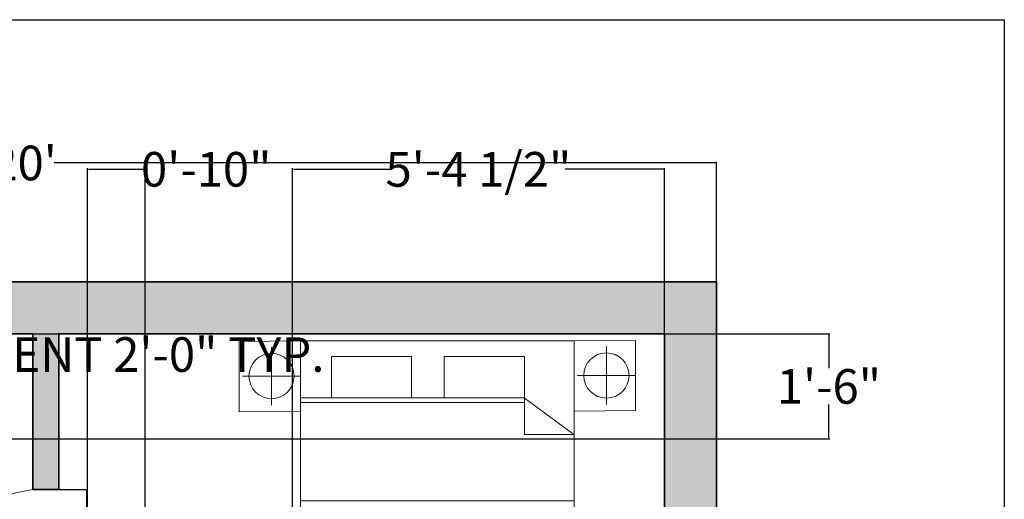
# Model space of a CAD drawing. Units: inches. Extents: x 335 to 688, y 1043 to 1486.
# Tile 7 of 7: x 510 to 681, y 1403 to 1486. Entities that reach past the tile are written whole.
import ezdxf

# ---------------------------------------------------------------- set-up
doc = ezdxf.new("R2010")
doc.units = ezdxf.units.IN
doc.header["$MEASUREMENT"] = 0
for name, color, linetype, lineweight in [('A-ANNO-DIMS', 2, 'Continuous', 18), ('A-ANNO-TTLB', 7, 'Continuous', 25), ('A-DOOR', 4, 'Continuous', 18), ('A-FURN', 8, 'Continuous', 18), ('A-WALL', 7, 'Continuous', 35), ('A-WALL-PATT', 252, 'Continuous', 13)]:
    doc.layers.add(name, color=color, linetype=linetype, lineweight=lineweight)
doc.styles.get("Standard").update_dxf_attribs({"font": 'arial.ttf'})
doc.dimstyles.get("Standard").update_dxf_attribs({"dimtxt": 6, "dimasz": 0.18, "dimexe": 0.18, "dimexo": 0.0625, "dimgap": 0.09, "dimtad": 0, "dimtih": 1, "dimtoh": 1, "dimdec": 1, "dimzin": 0, "dimdsep": 46, "dimlunit": 3, "dimtxsty": 'Standard', "dimcen": 0.09, "dimadec": 0, "dimazin": 0, "dimtfac": 1, "dimtdec": 1, "dimtofl": 0, "dimtmove": 0, "dimatfit": 3, "dimfxl": 1, "dimtolj": 1, "dimtzin": 0, "dimarcsym": 0})

# ---------------------------------------------------------------- blocks, each defined once
blk = doc.blocks.new('*D3')
at = {"layer": 'A-ANNO-DIMS', "color": 0, "lineweight": -2, "transparency": 16777216}
for p, q in [((391.11, 1441.03), (391.11, 1461.75)), ((391.29, 1461.57), (505.87, 1461.57)), ((630.93, 1461.57), (516.34, 1461.57)), ((631.11, 1441.03), (631.11, 1461.75))]:
    blk.add_line(p, q, dxfattribs=at)
at = {"layer": 'A-ANNO-DIMS', "color": 0, "transparency": 16777216}
for points in [[(391.29, 1461.6), (391.29, 1461.54), (391.11, 1461.57)], [(630.93, 1461.6), (630.93, 1461.54), (631.11, 1461.57)]]:
    blk.add_solid(points, dxfattribs=at)
at = {"layer": 'Defpoints', "color": 0, "transparency": 16777216}
for p in [(631.11, 1461.57), (391.11, 1440.97), (631.11, 1440.97)]:
    blk.add_point(p, dxfattribs=at)
at = {"layer": 'A-ANNO-DIMS', "color": 0, "transparency": 16777216, "insert": (511.11, 1461.57), "char_height": 6, "attachment_point": 5}
blk.add_mtext("\\A1;20'", dxfattribs=at)
blk = doc.blocks.new('BED-DOUBLE-WITH-NIGHTSTANDS')
for p, q in [((56.59, 58.08), (56.59, 68.14)), ((0, 64.35), (26.37, 64.35)), ((0, 1.12), (0, 64.35)), ((26.37, 64.35), (26.37, 58.06)), ((61.62, 63.11), (51.56, 63.11)), ((34.96, 10.66), (34.96, 58.08)), ((52, 19.27), (52, 58.08)), ((52.82, 19.32), (52.82, 58.08)), ((52.82, 19.32), (46.47, 10.71)), ((52.82, 19.27), (46.47, 19.27)), ((46.47, 19.27), (46.47, 10.71)), ((26.37, 10.66), (26.37, 1.12)), ((56.69, 0.03), (56.69, 10.09)), ((61.72, 5.06), (51.66, 5.06)), ((26.37, 1.12), (0, 1.12))]:
    blk.add_line(p, q)
for points in [[(50.39, 68.71), (50.5, 58.08), (62.68, 58.08), (62.58, 68.71)], [(62.68, 10.66), (11.37, 10.66), (11.37, 58.08), (62.68, 58.08)], [(59.98, 38.83), (52.82, 38.83), (52.82, 52.73), (59.98, 52.73)], [(59.98, 19.27), (52.82, 19.27), (52.82, 33.16), (59.98, 33.16)], [(50.5, 10.66), (50.6, 0.03), (62.78, 0.03), (62.68, 10.66)]]:
    blk.add_lwpolyline(points, close=True)
for centre in [(56.59, 63.11), (56.69, 5.06)]:
    blk.add_circle(centre, 3.92)
for points, knots in [([(0.07, 65.48), (0.19, 65.39), (0.43, 65.19), (0.19, 64.85), (0.02, 64.57), (0.13, 64.42), (0.18, 64.35)], [0, 0, 0, 0, 0.400747, 0.791423, 1.067667, 1.29709, 1.29709, 1.29709, 1.29709]), ([(0.57, 65.48), (0.7, 65.39), (0.94, 65.19), (0.7, 64.85), (0.52, 64.57), (0.63, 64.42), (0.68, 64.35)], [0, 0, 0, 0, 0.400747, 0.791423, 1.067667, 1.29709, 1.29709, 1.29709, 1.29709]), ([(1.06, 65.48), (1.18, 65.39), (1.42, 65.19), (1.18, 64.85), (1.01, 64.57), (1.11, 64.42), (1.16, 64.35)], [0, 0, 0, 0, 0.400747, 0.791423, 1.067667, 1.29709, 1.29709, 1.29709, 1.29709]), ([(1.46, 65.48), (1.58, 65.39), (1.82, 65.19), (1.58, 64.85), (1.41, 64.57), (1.51, 64.42), (1.56, 64.35)], [0, 0, 0, 0, 0.400747, 0.791423, 1.067667, 1.29709, 1.29709, 1.29709, 1.29709]), ([(1.88, 65.48), (2, 65.39), (2.24, 65.19), (2, 64.85), (1.82, 64.57), (1.93, 64.42), (1.98, 64.35)], [0, 0, 0, 0, 0.400747, 0.791423, 1.067667, 1.29709, 1.29709, 1.29709, 1.29709]), ([(2.18, 65.48), (2.31, 65.39), (2.55, 65.19), (2.31, 64.85), (2.13, 64.57), (2.24, 64.42), (2.29, 64.35)], [0, 0, 0, 0, 0.400747, 0.791423, 1.067667, 1.29709, 1.29709, 1.29709, 1.29709]), ([(2.76, 65.48), (2.88, 65.39), (3.12, 65.19), (2.88, 64.85), (2.71, 64.57), (2.81, 64.42), (2.86, 64.35)], [0, 0, 0, 0, 0.400747, 0.791423, 1.067667, 1.29709, 1.29709, 1.29709, 1.29709]), ([(3.33, 65.48), (3.45, 65.39), (3.7, 65.19), (3.44, 64.85), (3.27, 64.57), (3.38, 64.42), (3.43, 64.35)], [0, 0, 0, 0, 0.407265, 0.802015, 1.07826, 1.307683, 1.307683, 1.307683, 1.307683]), ([(3.75, 65.48), (3.88, 65.39), (4.12, 65.19), (3.88, 64.85), (3.7, 64.57), (3.81, 64.42), (3.86, 64.35)], [0, 0, 0, 0, 0.400747, 0.791423, 1.067667, 1.29709, 1.29709, 1.29709, 1.29709]), ([(4.64, 65.48), (4.76, 65.39), (5, 65.19), (4.76, 64.85), (4.59, 64.57), (4.69, 64.42), (4.74, 64.35)], [0, 0, 0, 0, 0.400747, 0.791423, 1.067667, 1.29709, 1.29709, 1.29709, 1.29709]), ([(5.36, 65.48), (5.49, 65.39), (5.73, 65.19), (5.49, 64.85), (5.31, 64.57), (5.42, 64.42), (5.47, 64.35)], [0, 0, 0, 0, 0.400747, 0.791423, 1.067667, 1.29709, 1.29709, 1.29709, 1.29709]), ([(6.12, 65.48), (6.24, 65.39), (6.48, 65.19), (6.24, 64.85), (6.07, 64.57), (6.17, 64.42), (6.22, 64.35)], [0, 0, 0, 0, 0.400747, 0.791423, 1.067667, 1.29709, 1.29709, 1.29709, 1.29709]), ([(7, 65.48), (7.12, 65.39), (7.36, 65.19), (7.12, 64.85), (6.95, 64.57), (7.05, 64.42), (7.1, 64.35)], [0, 0, 0, 0, 0.400747, 0.791423, 1.067667, 1.29709, 1.29709, 1.29709, 1.29709]), ([(7.73, 65.48), (7.85, 65.39), (8.09, 65.19), (7.85, 64.85), (7.68, 64.57), (7.78, 64.42), (7.83, 64.35)], [0, 0, 0, 0, 0.400747, 0.791423, 1.067667, 1.29709, 1.29709, 1.29709, 1.29709]), ([(8.54, 65.48), (8.66, 65.39), (8.9, 65.19), (8.66, 64.85), (8.49, 64.57), (8.6, 64.42), (8.65, 64.35)], [0, 0, 0, 0, 0.400747, 0.791423, 1.067667, 1.29709, 1.29709, 1.29709, 1.29709]), ([(9.23, 65.48), (9.35, 65.39), (9.59, 65.19), (9.35, 64.85), (9.18, 64.57), (9.29, 64.42), (9.34, 64.35)], [0, 0, 0, 0, 0.400747, 0.791423, 1.067667, 1.29709, 1.29709, 1.29709, 1.29709]), ([(10.05, 65.48), (10.17, 65.39), (10.41, 65.19), (10.17, 64.85), (10, 64.57), (10.1, 64.42), (10.15, 64.35)], [0, 0, 0, 0, 0.400747, 0.791423, 1.067667, 1.29709, 1.29709, 1.29709, 1.29709]), ([(10.93, 65.48), (11.05, 65.39), (11.29, 65.19), (11.05, 64.85), (10.88, 64.57), (10.99, 64.42), (11.03, 64.35)], [0, 0, 0, 0, 0.400747, 0.791423, 1.067667, 1.29709, 1.29709, 1.29709, 1.29709]), ([(11.97, 65.48), (12.09, 65.39), (12.33, 65.19), (12.09, 64.85), (11.92, 64.57), (12.02, 64.42), (12.07, 64.35)], [0, 0, 0, 0, 0.400747, 0.791423, 1.067667, 1.29709, 1.29709, 1.29709, 1.29709]), ([(12.85, 65.48), (12.97, 65.39), (13.21, 65.19), (12.97, 64.85), (12.8, 64.57), (12.9, 64.42), (12.95, 64.35)], [0, 0, 0, 0, 0.400747, 0.791423, 1.067667, 1.29709, 1.29709, 1.29709, 1.29709]), ([(13.58, 65.48), (13.7, 65.39), (13.94, 65.19), (13.7, 64.85), (13.53, 64.57), (13.63, 64.42), (13.68, 64.35)], [0, 0, 0, 0, 0.400747, 0.791423, 1.067667, 1.29709, 1.29709, 1.29709, 1.29709]), ([(14.33, 65.48), (14.45, 65.39), (14.69, 65.19), (14.45, 64.85), (14.28, 64.57), (14.38, 64.42), (14.43, 64.35)], [0, 0, 0, 0, 0.400747, 0.791423, 1.067667, 1.29709, 1.29709, 1.29709, 1.29709]), ([(15.21, 65.48), (15.33, 65.39), (15.57, 65.19), (15.33, 64.85), (15.16, 64.57), (15.27, 64.42), (15.32, 64.35)], [0, 0, 0, 0, 0.400747, 0.791423, 1.067667, 1.29709, 1.29709, 1.29709, 1.29709]), ([(15.94, 65.48), (16.06, 65.39), (16.3, 65.19), (16.06, 64.85), (15.89, 64.57), (16, 64.42), (16.04, 64.35)], [0, 0, 0, 0, 0.400747, 0.791423, 1.067667, 1.29709, 1.29709, 1.29709, 1.29709]), ([(16.76, 65.48), (16.88, 65.39), (17.12, 65.19), (16.88, 64.85), (16.7, 64.57), (16.81, 64.42), (16.86, 64.35)], [0, 0, 0, 0, 0.400747, 0.791423, 1.067667, 1.29709, 1.29709, 1.29709, 1.29709]), ([(17.53, 65.48), (17.65, 65.39), (17.89, 65.19), (17.65, 64.85), (17.48, 64.57), (17.59, 64.42), (17.64, 64.35)], [0, 0, 0, 0, 0.400747, 0.791423, 1.067667, 1.29709, 1.29709, 1.29709, 1.29709]), ([(18.35, 65.48), (18.47, 65.39), (18.71, 65.19), (18.47, 64.85), (18.3, 64.57), (18.4, 64.42), (18.45, 64.35)], [0, 0, 0, 0, 0.400747, 0.791423, 1.067667, 1.29709, 1.29709, 1.29709, 1.29709]), ([(19.23, 65.48), (19.35, 65.39), (19.59, 65.19), (19.35, 64.85), (19.18, 64.57), (19.29, 64.42), (19.33, 64.35)], [0, 0, 0, 0, 0.400747, 0.791423, 1.067667, 1.29709, 1.29709, 1.29709, 1.29709]), ([(20.27, 65.48), (20.39, 65.39), (20.63, 65.19), (20.39, 64.85), (20.22, 64.57), (20.32, 64.42), (20.37, 64.35)], [0, 0, 0, 0, 0.400747, 0.791423, 1.067667, 1.29709, 1.29709, 1.29709, 1.29709]), ([(21.15, 65.48), (21.27, 65.39), (21.51, 65.19), (21.27, 64.85), (21.1, 64.57), (21.21, 64.42), (21.25, 64.35)], [0, 0, 0, 0, 0.400747, 0.791423, 1.067667, 1.29709, 1.29709, 1.29709, 1.29709]), ([(21.88, 65.48), (22, 65.39), (22.24, 65.19), (22, 64.85), (21.83, 64.57), (21.93, 64.42), (21.98, 64.35)], [0, 0, 0, 0, 0.400747, 0.791423, 1.067667, 1.29709, 1.29709, 1.29709, 1.29709]), ([(22.63, 65.48), (22.75, 65.39), (22.99, 65.19), (22.75, 64.85), (22.58, 64.57), (22.69, 64.42), (22.73, 64.35)], [0, 0, 0, 0, 0.400747, 0.791423, 1.067667, 1.29709, 1.29709, 1.29709, 1.29709]), ([(23.51, 65.48), (23.63, 65.39), (23.87, 65.19), (23.63, 64.85), (23.46, 64.57), (23.57, 64.42), (23.62, 64.35)], [0, 0, 0, 0, 0.400747, 0.791423, 1.067667, 1.29709, 1.29709, 1.29709, 1.29709]), ([(24.24, 65.48), (24.36, 65.39), (24.6, 65.19), (24.36, 64.85), (24.19, 64.57), (24.3, 64.42), (24.34, 64.35)], [0, 0, 0, 0, 0.400747, 0.791423, 1.067667, 1.29709, 1.29709, 1.29709, 1.29709]), ([(25.06, 65.48), (25.18, 65.39), (25.42, 65.19), (25.18, 64.85), (25.01, 64.57), (25.11, 64.42), (25.16, 64.35)], [0, 0, 0, 0, 0.400747, 0.791423, 1.067667, 1.29709, 1.29709, 1.29709, 1.29709]), ([(25.84, 65.48), (25.96, 65.39), (26.2, 65.19), (25.96, 64.85), (25.78, 64.57), (25.89, 64.42), (25.94, 64.35)], [0, 0, 0, 0, 0.400747, 0.791423, 1.067667, 1.29709, 1.29709, 1.29709, 1.29709]), ([(0.07, 0), (0.19, 0.1), (0.43, 0.29), (0.19, 0.63), (0.02, 0.91), (0.13, 1.06), (0.18, 1.13)], [0, 0, 0, 0, 0.400747, 0.791423, 1.067667, 1.29709, 1.29709, 1.29709, 1.29709]), ([(0.55, 0), (0.67, 0.1), (0.91, 0.29), (0.67, 0.63), (0.49, 0.91), (0.6, 1.06), (0.65, 1.13)], [0, 0, 0, 0, 0.400747, 0.791423, 1.067667, 1.29709, 1.29709, 1.29709, 1.29709]), ([(1.03, 0), (1.15, 0.1), (1.39, 0.29), (1.15, 0.63), (0.98, 0.91), (1.09, 1.06), (1.13, 1.13)], [0, 0, 0, 0, 0.400747, 0.791423, 1.067667, 1.29709, 1.29709, 1.29709, 1.29709]), ([(1.43, 0), (1.55, 0.1), (1.79, 0.29), (1.55, 0.63), (1.38, 0.91), (1.48, 1.06), (1.53, 1.13)], [0, 0, 0, 0, 0.400747, 0.791423, 1.067667, 1.29709, 1.29709, 1.29709, 1.29709]), ([(1.85, 0), (1.97, 0.1), (2.21, 0.29), (1.97, 0.63), (1.8, 0.91), (1.9, 1.05), (1.94, 1.12)], [0, 0, 0, 0, 0.400747, 0.791423, 1.067667, 1.283686, 1.283686, 1.283686, 1.283686]), ([(2.16, 0), (2.28, 0.1), (2.52, 0.29), (2.28, 0.63), (2.11, 0.91), (2.21, 1.05), (2.25, 1.12)], [0, 0, 0, 0, 0.400747, 0.791423, 1.067667, 1.283686, 1.283686, 1.283686, 1.283686]), ([(2.73, 0), (2.85, 0.1), (3.09, 0.29), (2.85, 0.63), (2.68, 0.91), (2.78, 1.05), (2.82, 1.12)], [0, 0, 0, 0, 0.400747, 0.791423, 1.067667, 1.283686, 1.283686, 1.283686, 1.283686]), ([(3.33, 0), (3.45, 0.1), (3.69, 0.29), (3.45, 0.63), (3.28, 0.91), (3.38, 1.05), (3.42, 1.12)], [0, 0, 0, 0, 0.402903, 0.794912, 1.071156, 1.287177, 1.287177, 1.287177, 1.287177]), ([(3.75, 0), (3.88, 0.1), (4.12, 0.29), (3.88, 0.63), (3.7, 0.91), (3.81, 1.05), (3.85, 1.12)], [0, 0, 0, 0, 0.400747, 0.791423, 1.067667, 1.283686, 1.283686, 1.283686, 1.283686]), ([(4.64, 0), (4.76, 0.1), (5, 0.29), (4.76, 0.63), (4.59, 0.91), (4.69, 1.05), (4.73, 1.12)], [0, 0, 0, 0, 0.400747, 0.791423, 1.067667, 1.283686, 1.283686, 1.283686, 1.283686]), ([(5.36, 0), (5.49, 0.1), (5.73, 0.29), (5.49, 0.63), (5.31, 0.91), (5.42, 1.06), (5.47, 1.13)], [0, 0, 0, 0, 0.400747, 0.791423, 1.067667, 1.29709, 1.29709, 1.29709, 1.29709]), ([(6.12, 0), (6.24, 0.1), (6.48, 0.29), (6.24, 0.63), (6.07, 0.91), (6.17, 1.06), (6.22, 1.13)], [0, 0, 0, 0, 0.400747, 0.791423, 1.067667, 1.29709, 1.29709, 1.29709, 1.29709]), ([(7, 0), (7.12, 0.1), (7.36, 0.29), (7.12, 0.63), (6.95, 0.91), (7.05, 1.06), (7.1, 1.13)], [0, 0, 0, 0, 0.400747, 0.791423, 1.067667, 1.29709, 1.29709, 1.29709, 1.29709]), ([(7.73, 0), (7.85, 0.1), (8.09, 0.29), (7.85, 0.63), (7.68, 0.91), (7.78, 1.06), (7.83, 1.13)], [0, 0, 0, 0, 0.400747, 0.791423, 1.067667, 1.29709, 1.29709, 1.29709, 1.29709]), ([(8.54, 0), (8.66, 0.1), (8.9, 0.29), (8.66, 0.63), (8.49, 0.91), (8.6, 1.06), (8.65, 1.13)], [0, 0, 0, 0, 0.400747, 0.791423, 1.067667, 1.29709, 1.29709, 1.29709, 1.29709]), ([(9.23, 0), (9.35, 0.1), (9.59, 0.29), (9.35, 0.63), (9.18, 0.91), (9.29, 1.06), (9.34, 1.13)], [0, 0, 0, 0, 0.400747, 0.791423, 1.067667, 1.29709, 1.29709, 1.29709, 1.29709]), ([(10.05, 0), (10.17, 0.1), (10.41, 0.29), (10.17, 0.63), (10, 0.91), (10.1, 1.06), (10.15, 1.13)], [0, 0, 0, 0, 0.400747, 0.791423, 1.067667, 1.29709, 1.29709, 1.29709, 1.29709]), ([(10.93, 0), (11.05, 0.1), (11.29, 0.29), (11.05, 0.63), (10.88, 0.91), (10.99, 1.06), (11.03, 1.13)], [0, 0, 0, 0, 0.400747, 0.791423, 1.067667, 1.29709, 1.29709, 1.29709, 1.29709]), ([(11.97, 0), (12.09, 0.1), (12.33, 0.29), (12.09, 0.63), (11.92, 0.91), (12.02, 1.06), (12.07, 1.13)], [0, 0, 0, 0, 0.400747, 0.791423, 1.067667, 1.29709, 1.29709, 1.29709, 1.29709]), ([(12.85, 0), (12.97, 0.1), (13.21, 0.29), (12.97, 0.63), (12.8, 0.91), (12.9, 1.06), (12.95, 1.13)], [0, 0, 0, 0, 0.400747, 0.791423, 1.067667, 1.29709, 1.29709, 1.29709, 1.29709]), ([(13.58, 0), (13.7, 0.1), (13.94, 0.29), (13.7, 0.63), (13.53, 0.91), (13.63, 1.06), (13.68, 1.13)], [0, 0, 0, 0, 0.400747, 0.791423, 1.067667, 1.29709, 1.29709, 1.29709, 1.29709]), ([(14.33, 0), (14.45, 0.1), (14.69, 0.29), (14.45, 0.63), (14.28, 0.91), (14.38, 1.06), (14.43, 1.13)], [0, 0, 0, 0, 0.400747, 0.791423, 1.067667, 1.29709, 1.29709, 1.29709, 1.29709]), ([(15.21, 0), (15.33, 0.1), (15.57, 0.29), (15.33, 0.63), (15.16, 0.91), (15.27, 1.06), (15.32, 1.13)], [0, 0, 0, 0, 0.400747, 0.791423, 1.067667, 1.29709, 1.29709, 1.29709, 1.29709]), ([(15.94, 0), (16.06, 0.1), (16.3, 0.29), (16.06, 0.63), (15.89, 0.91), (16, 1.06), (16.04, 1.13)], [0, 0, 0, 0, 0.400747, 0.791423, 1.067667, 1.29709, 1.29709, 1.29709, 1.29709]), ([(16.76, 0), (16.88, 0.1), (17.12, 0.29), (16.88, 0.63), (16.7, 0.91), (16.81, 1.06), (16.86, 1.13)], [0, 0, 0, 0, 0.400747, 0.791423, 1.067667, 1.29709, 1.29709, 1.29709, 1.29709]), ([(17.53, 0), (17.65, 0.1), (17.89, 0.29), (17.65, 0.63), (17.48, 0.91), (17.59, 1.06), (17.64, 1.13)], [0, 0, 0, 0, 0.400747, 0.791423, 1.067667, 1.29709, 1.29709, 1.29709, 1.29709]), ([(18.35, 0), (18.47, 0.1), (18.71, 0.29), (18.47, 0.63), (18.3, 0.91), (18.4, 1.06), (18.45, 1.13)], [0, 0, 0, 0, 0.400747, 0.791423, 1.067667, 1.29709, 1.29709, 1.29709, 1.29709]), ([(19.23, 0), (19.35, 0.1), (19.59, 0.29), (19.35, 0.63), (19.18, 0.91), (19.29, 1.06), (19.33, 1.13)], [0, 0, 0, 0, 0.400747, 0.791423, 1.067667, 1.29709, 1.29709, 1.29709, 1.29709]), ([(20.27, 0), (20.39, 0.1), (20.63, 0.29), (20.39, 0.63), (20.22, 0.91), (20.32, 1.06), (20.37, 1.13)], [0, 0, 0, 0, 0.400747, 0.791423, 1.067667, 1.29709, 1.29709, 1.29709, 1.29709]), ([(21.15, 0), (21.27, 0.1), (21.51, 0.29), (21.27, 0.63), (21.1, 0.91), (21.21, 1.06), (21.25, 1.13)], [0, 0, 0, 0, 0.400747, 0.791423, 1.067667, 1.29709, 1.29709, 1.29709, 1.29709]), ([(21.88, 0), (22, 0.1), (22.24, 0.29), (22, 0.63), (21.83, 0.91), (21.93, 1.06), (21.98, 1.13)], [0, 0, 0, 0, 0.400747, 0.791423, 1.067667, 1.29709, 1.29709, 1.29709, 1.29709]), ([(22.63, 0), (22.75, 0.1), (22.99, 0.29), (22.75, 0.63), (22.58, 0.91), (22.69, 1.06), (22.73, 1.13)], [0, 0, 0, 0, 0.400747, 0.791423, 1.067667, 1.29709, 1.29709, 1.29709, 1.29709]), ([(23.51, 0), (23.63, 0.1), (23.87, 0.29), (23.63, 0.63), (23.46, 0.91), (23.57, 1.06), (23.62, 1.13)], [0, 0, 0, 0, 0.400747, 0.791423, 1.067667, 1.29709, 1.29709, 1.29709, 1.29709]), ([(24.24, 0), (24.36, 0.1), (24.6, 0.29), (24.36, 0.63), (24.19, 0.91), (24.3, 1.06), (24.34, 1.13)], [0, 0, 0, 0, 0.400747, 0.791423, 1.067667, 1.29709, 1.29709, 1.29709, 1.29709]), ([(25.06, 0), (25.18, 0.1), (25.42, 0.29), (25.18, 0.63), (25.01, 0.91), (25.11, 1.06), (25.16, 1.13)], [0, 0, 0, 0, 0.400747, 0.791423, 1.067667, 1.29709, 1.29709, 1.29709, 1.29709]), ([(25.84, 0), (25.96, 0.1), (26.2, 0.29), (25.96, 0.63), (25.78, 0.91), (25.89, 1.06), (25.94, 1.13)], [0, 0, 0, 0, 0.400747, 0.791423, 1.067667, 1.29709, 1.29709, 1.29709, 1.29709])]:
    blk.add_open_spline(points, degree=3, knots=knots)
blk = doc.blocks.new('DOOR-32IN')
for p, q in [((0, 1), (32, 1)), ((32, 0), (32, 1)), ((32, 0), (0, 0)), ((0, 0), (32, 0))]:
    blk.add_line(p, q)
blk.add_arc((32.37, 0), 32.37, 98.6501, 180)
blk = doc.blocks.new('*D27')
at = {"layer": 'A-ANNO-DIMS', "color": 0, "lineweight": -2, "transparency": 16777216}
for p, q in [((478.71, 1431.9), (478.71, 1428.19)), ((502.71, 1431.9), (502.71, 1428.19)), ((478.89, 1428.37), (502.53, 1428.37)), ((502.71, 1428.37), (502.89, 1428.37))]:
    blk.add_line(p, q, dxfattribs=at)
at = {"layer": 'A-ANNO-DIMS', "color": 0, "transparency": 16777216}
for points in [[(478.89, 1428.4), (478.89, 1428.34), (478.71, 1428.37)], [(502.53, 1428.4), (502.53, 1428.34), (502.71, 1428.37)]]:
    blk.add_solid(points, dxfattribs=at)
at = {"layer": 'Defpoints', "color": 0, "transparency": 16777216}
for p in [(478.71, 1431.97), (502.71, 1431.97), (502.71, 1428.37)]:
    blk.add_point(p, dxfattribs=at)
at = {"layer": 'A-ANNO-DIMS', "color": 0, "transparency": 16777216, "insert": (533.76, 1428.37), "char_height": 6, "attachment_point": 5}
blk.add_mtext('\\A1;VENT 2\'-0" TYP.', dxfattribs=at)
blk = doc.blocks.new('*D30')
at = {"layer": 'A-ANNO-DIMS', "color": 0, "lineweight": -2, "transparency": 16777216}
for p, q in [((517.17, 1404.97), (522.09, 1404.97)), ((521.91, 1404.79), (521.91, 1392.12)), ((521.91, 1373.15), (521.91, 1385.81)), ((517.17, 1372.97), (522.09, 1372.97))]:
    blk.add_line(p, q, dxfattribs=at)
at = {"layer": 'A-ANNO-DIMS', "color": 0, "transparency": 16777216}
for points in [[(521.88, 1404.79), (521.94, 1404.79), (521.91, 1404.97)], [(521.88, 1373.15), (521.94, 1373.15), (521.91, 1372.97)]]:
    blk.add_solid(points, dxfattribs=at)
at = {"layer": 'Defpoints', "color": 0, "transparency": 16777216}
for p in [(517.11, 1404.97), (521.91, 1404.97), (517.11, 1372.97)]:
    blk.add_point(p, dxfattribs=at)
at = {"layer": 'A-ANNO-DIMS', "color": 0, "transparency": 16777216, "insert": (521.91, 1388.97), "char_height": 6, "attachment_point": 5}
blk.add_mtext('\\A1;2\'-8" TYP.', dxfattribs=at)
blk = doc.blocks.new('*D42')
at = {"layer": 'A-ANNO-DIMS', "color": 0, "lineweight": -2, "transparency": 16777216}
for p, q in [((557.61, 1309.03), (557.61, 1460.65)), ((557.79, 1460.47), (574.8, 1460.47)), ((621.93, 1460.47), (604.91, 1460.47)), ((622.11, 1309.03), (622.11, 1460.65))]:
    blk.add_line(p, q, dxfattribs=at)
at = {"layer": 'A-ANNO-DIMS', "color": 0, "transparency": 16777216}
for points in [[(557.79, 1460.5), (557.79, 1460.44), (557.61, 1460.47)], [(621.93, 1460.5), (621.93, 1460.44), (622.11, 1460.47)]]:
    blk.add_solid(points, dxfattribs=at)
at = {"layer": 'Defpoints', "color": 0, "transparency": 16777216}
for p in [(622.11, 1460.47), (557.61, 1308.97), (622.11, 1308.97)]:
    blk.add_point(p, dxfattribs=at)
at = {"layer": 'A-ANNO-DIMS', "color": 0, "transparency": 16777216, "insert": (589.86, 1460.47), "char_height": 6, "attachment_point": 5}
blk.add_mtext('\\A1;5\'-4 1/2"', dxfattribs=at)
blk = doc.blocks.new('*D57')
at = {"layer": 'A-ANNO-DIMS', "color": 0, "lineweight": -2, "transparency": 16777216}
for p, q in [((522.11, 1090.03), (522.11, 1460.65)), ((522.29, 1460.47), (531.93, 1460.47)), ((532.11, 1090.03), (532.11, 1460.65)), ((532.11, 1460.47), (532.29, 1460.47))]:
    blk.add_line(p, q, dxfattribs=at)
at = {"layer": 'A-ANNO-DIMS', "color": 0, "transparency": 16777216}
for points in [[(522.29, 1460.5), (522.29, 1460.44), (522.11, 1460.47)], [(531.93, 1460.5), (531.93, 1460.44), (532.11, 1460.47)]]:
    blk.add_solid(points, dxfattribs=at)
at = {"layer": 'Defpoints', "color": 0, "transparency": 16777216}
for p in [(532.11, 1460.47), (522.11, 1089.97), (532.11, 1089.97)]:
    blk.add_point(p, dxfattribs=at)
at = {"layer": 'A-ANNO-DIMS', "color": 0, "transparency": 16777216, "insert": (542.68, 1460.47), "char_height": 6, "attachment_point": 5}
blk.add_mtext('\\A1;0\'-10"', dxfattribs=at)
blk = doc.blocks.new('*D63')
at = {"layer": 'A-ANNO-DIMS', "color": 0, "lineweight": -2, "transparency": 16777216}
for p, q in [((466.17, 1431.97), (650.79, 1431.97)), ((650.61, 1431.79), (650.61, 1426.01)), ((650.61, 1413.92), (650.61, 1419.7)), ((466.17, 1413.74), (650.79, 1413.74))]:
    blk.add_line(p, q, dxfattribs=at)
at = {"layer": 'A-ANNO-DIMS', "color": 0, "transparency": 16777216}
for points in [[(650.58, 1431.79), (650.64, 1431.79), (650.61, 1431.97)], [(650.58, 1413.92), (650.64, 1413.92), (650.61, 1413.74)]]:
    blk.add_solid(points, dxfattribs=at)
at = {"layer": 'Defpoints', "color": 0, "transparency": 16777216}
for p in [(466.11, 1431.97), (650.61, 1431.97), (466.11, 1413.74)]:
    blk.add_point(p, dxfattribs=at)
at = {"layer": 'A-ANNO-DIMS', "color": 0, "transparency": 16777216, "insert": (650.61, 1422.85), "char_height": 6, "attachment_point": 5}
blk.add_mtext('\\A1;1\'-6"', dxfattribs=at)

msp = doc.modelspace()

# ---------------------------------------------------------------- hatches: boundary and pattern name
at = {"layer": 'A-WALL-PATT'}
h = msp.add_hatch(color=256, dxfattribs=at)
h.dxf.hatch_style = 1
h.paths.add_polyline_path([(478.71, 1440.97), (391.11, 1440.97), (391.11, 1411.42), (400.11, 1411.42), (400.11, 1431.97), (466.11, 1431.97), (466.11, 1347.97), (466.11, 1343.47), (470.61, 1343.47), (470.61, 1367.47), (512.61, 1367.47), (512.61, 1350.97), (517.11, 1350.97), (517.11, 1372.97), (512.61, 1372.97), (512.61, 1371.97), (470.61, 1371.97), (470.61, 1431.97), (478.71, 1431.97)])
h.paths.add_polyline_path([(631.11, 1440.97), (502.71, 1440.97), (502.71, 1431.97), (512.61, 1431.97), (512.61, 1404.97), (517.11, 1404.97), (517.11, 1431.97), (622.11, 1431.97), (622.11, 1401.6), (631.11, 1401.6)])
h.paths.add_polyline_path([(631.11, 1341.6), (622.11, 1341.6), (622.11, 1313.47), (517.11, 1313.47), (517.11, 1314.47), (512.61, 1314.47), (512.61, 1313.47), (512.61, 1307.97), (517.11, 1307.97), (517.11, 1308.97), (553.11, 1308.97), (553.11, 1262.47), (558.61, 1262.47), (558.61, 1266.97), (557.61, 1266.97), (557.61, 1308.97), (622.11, 1308.97), (622.11, 1297.63), (631.11, 1297.63)])
h.paths.add_polyline_path([(631.11, 1273.63), (622.11, 1273.63), (622.11, 1266.97), (590.61, 1266.97), (590.61, 1262.47), (622.11, 1262.47), (622.11, 1230.86), (631.11, 1230.86)])
h.paths.add_polyline_path([(400.11, 1253.85), (391.11, 1253.85), (391.11, 1132.26), (400.11, 1132.26), (400.11, 1149.97), (411.11, 1149.97), (411.11, 1154.47), (400.11, 1154.47)], flags=17)
h.paths.add_polyline_path([(400.11, 1375.42), (391.11, 1375.42), (391.11, 1313.85), (400.11, 1313.85), (400.11, 1343.47), (428.36, 1343.47), (428.36, 1347.97), (400.11, 1347.97)])

# ---------------------------------------------------------------- linework, layer by layer
at = {"layer": 'A-ANNO-TTLB'}
msp.add_lwpolyline([(334.72, 1486.4), (681.01, 1486.4), (681.01, 1043.03), (334.72, 1043.03)], close=True, dxfattribs=at)
at = {"layer": 'A-WALL'}
for p, q in [((391.11, 1440.97), (631.11, 1440.97)), ((631.11, 1440.97), (631.11, 1080.97)), ((470.61, 1431.97), (512.61, 1431.97)), ((512.61, 1431.97), (512.61, 1404.97)), ((517.11, 1431.97), (517.11, 1404.97)), ((517.11, 1431.97), (622.11, 1431.97)), ((622.11, 1431.97), (622.11, 1313.47)), ((517.11, 1404.97), (512.61, 1404.97))]:
    msp.add_line(p, q, dxfattribs=at)

# ---------------------------------------------------------------- block references
at = {"layer": 'A-DOOR'}
msp.add_blockref('DOOR-32IN', (485.11, 1372.97), dxfattribs=at)
at = {"layer": 'A-FURN', "rotation": 89.99999999999726}
msp.add_blockref('BED-DOUBLE-WITH-NIGHTSTANDS', (617.1, 1368.05), dxfattribs=at)

# ---------------------------------------------------------------- dimensions: what is measured, and where the dimension line sits
at = {"layer": 'A-ANNO-DIMS'}
for base, p1, p2, override, picture, middle in [((622.11, 1460.47), (557.61, 1308.97), (622.11, 1308.97), {"dimdec": 1, "dimlfac": 1, "dimrnd": 0, "dimzin": 1, "dimdsep": 46, "dimlunit": 4, "dimfrac": 2}, '*D42', (589.86, 1460.47)), ((631.11, 1461.57), (391.11, 1440.97), (631.11, 1440.97), {"dimclrd": 0, "dimclre": 0, "dimclrt": 0}, '*D3', (511.11, 1461.57)), ((532.11, 1460.47), (522.11, 1089.97), (532.11, 1089.97), {"dimdec": 1, "dimlfac": 1, "dimrnd": 0, "dimzin": 1, "dimdsep": 46, "dimlunit": 4, "dimfrac": 2}, '*D57', (542.68, 1460.47))]:
    dim = msp.add_linear_dim(base=base, p1=p1, p2=p2, dimstyle='Standard', override=override, dxfattribs=at)
    dim.commit()
    dim.dimension.update_dxf_attribs({"geometry": picture, "text_midpoint": middle})
dim = msp.add_linear_dim(base=(502.71, 1428.37), p1=(478.71, 1431.97), p2=(502.71, 1431.97), text='VENT <> TYP.', dimstyle='Standard', override={"dimdec": 1, "dimlfac": 1, "dimrnd": 0, "dimzin": 1, "dimdsep": 46, "dimlunit": 4, "dimfrac": 2}, dxfattribs=at)
dim.commit()
dim.dimension.update_dxf_attribs({"geometry": '*D27', "text_midpoint": (533.76, 1428.37)})
dim = msp.add_linear_dim(base=(650.61, 1431.97), p1=(466.11, 1413.74), p2=(466.11, 1431.97), angle=90, dimstyle='Standard', override={"dimdec": 1, "dimlfac": 1, "dimrnd": 0, "dimzin": 1, "dimdsep": 46, "dimlunit": 4, "dimfrac": 2}, dxfattribs=at)
dim.commit()
dim.dimension.update_dxf_attribs({"geometry": '*D63', "text_midpoint": (650.61, 1422.85)})
dim = msp.add_linear_dim(base=(521.91, 1404.97), p1=(517.11, 1372.97), p2=(517.11, 1404.97), angle=90, text='<> TYP.', dimstyle='Standard', override={"dimdec": 1, "dimlfac": 1, "dimrnd": 0, "dimzin": 1, "dimdsep": 46, "dimlunit": 4, "dimfrac": 2}, dxfattribs=at)
dim.commit()
dim.dimension.update_dxf_attribs({"geometry": '*D30', "text_midpoint": (521.91, 1388.97)})

doc.saveas('drawing.dxf')
